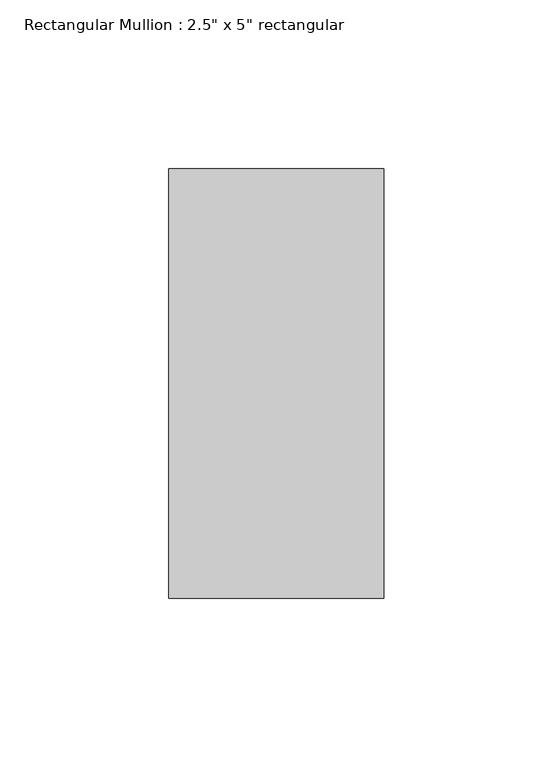
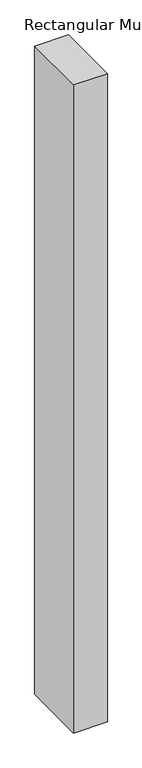
"""IFC4 building model written with IfcOpenShell, lengths in millimetres: member geometry."""

from ifc_helpers import new_model, si_unit, frame, origin, place, context, project, spatial, polyline, outline, extrude, source, transform, mapped, element, save


def member_bf3bc0fd(model_context):
    return source(origin(), model_context, "Body", "SweptSolid", [
        extrude(outline(polyline([(0.0, 63.5), (0.0, -63.5), (-63.5, -63.5), (-63.5, 63.5), (0.0, 63.5)])), frame((0.0, 0.0, -1291.1666667), z_axis=(0.0, 0.0, 1.0), x_axis=(1.0, 0.0, 0.0)), (0.0, 0.0, 1.0), 1291.1666667),
    ])


if __name__ == "__main__":
    model = new_model("IFC4")
    model_context = context("Model", 3, world=origin())
    ifc_project = project(units=[si_unit("LENGTHUNIT", "METRE", prefix="MILLI")], contexts=[model_context])
    site = spatial("IfcSite", under=ifc_project)
    building = spatial("IfcBuilding", under=site)
    placement = place(None, origin())
    member_shape = member_bf3bc0fd(model_context)
    element("IfcMember", 1, ObjectType="Rectangular Mullion : 2.5\" x 5\" rectangular", at=placement, inside=building, context=model_context, shape_type="MappedRepresentation", body=[
        mapped(member_shape, transform((0.0, 0.0, 0.0), x_axis=(1.0, 0.0, 0.0), y_axis=(0.0, 1.0, 0.0), z_axis=(0.0, 0.0, 1.0))),
    ])
    save(model, "model.ifc")

# Revit data of these elements
# Type "Rectangular Mullion : 2.5\" x 5\" rectangular"
#   built-in parameter 1007304 = 0.416667 (stored number, unit not read)
#   built-in parameter 1007301 = 0.104167 (stored number, unit not read)
#   built-in parameter 1007300 = 0.104167 (stored number, unit not read)
# Element 1 (IfcMember, "Rectangular Mullion : 2.5\" x 5\" rectangular")
#   Materials on its faces: "Aluminum"
# Materials
#   "Aluminum": class "Metal", colour RGB 247 247 247, transparency 0, Description = "Aluminum 6061", Cost = 0
